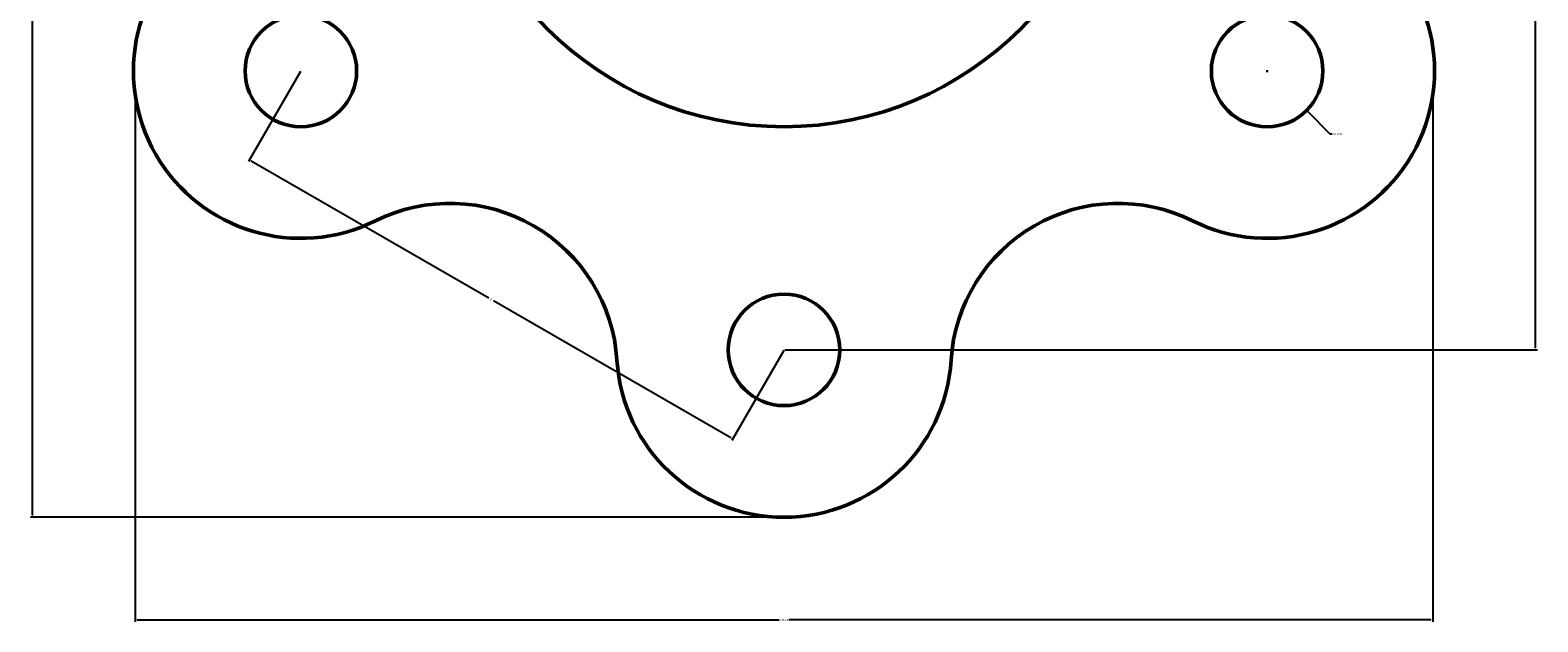
# Model space of a CAD drawing. Units: millimetres. Extents: x 2038 to 2173, y 1596 to 1745.
# Tile 1 of 4: x 2038 to 2173, y 1596 to 1649. Entities that reach past the tile are written whole.
import ezdxf

# ---------------------------------------------------------------- set-up
doc = ezdxf.new("R2010")
doc.units = ezdxf.units.MM
doc.layers.add('M-DIMS', color=2, linetype='Continuous', lineweight=18)
doc.layers.add('M-OUTL', color=7, linetype='Continuous', lineweight=50)
doc.styles.get("Standard").update_dxf_attribs({"font": 'arial.ttf'})
doc.dimstyles.get("Standard").update_dxf_attribs({"dimtxt": 0.18, "dimasz": 0.18, "dimexe": 0.18, "dimexo": 0.0625, "dimgap": 0.09, "dimtad": 0, "dimtih": 1, "dimtoh": 1, "dimdec": 4, "dimzin": 0, "dimdsep": 46, "dimtxsty": 'Standard', "dimcen": 0.09, "dimadec": 0, "dimazin": 0, "dimtfac": 1, "dimtdec": 4, "dimtofl": 0, "dimtmove": 0, "dimatfit": 3, "dimfxl": 1, "dimtolj": 1, "dimtzin": 0, "dimarcsym": 0})

# ---------------------------------------------------------------- blocks, each defined once
blk = doc.blocks.new('*U1')
blk.add_arc((-4.15, 7.97), 15, 243.5573, 356.4427)
blk = doc.blocks.new('*U2')
at = {"layer": 'M-OUTL', "color": 0, "linetype": 'ByBlock', "lineweight": -2, "transparency": 16777216}
for p, rotation in [((2130.6, 1715.07), 300), ((2156.4, 1671.18), 240), ((2054.57, 1670.39), 60.00000000000003), ((2080.37, 1626.5), 120.0000000000001), ((2131.28, 1626.89), 180)]:
    blk.add_blockref('*U1', p, dxfattribs=dict(at, rotation=rotation))
blk.add_blockref('*U1', (2079.69, 1714.68), dxfattribs=at)
blk = doc.blocks.new('FLANGE-LUG-D10')
blk.add_circle((0, 0), 5)
blk.add_arc((0, 0), 15, 3.5573, 176.4427)
blk = doc.blocks.new('*D4')
at = {"layer": 'Defpoints', "color": 0, "transparency": 16777216}
for p in [(2047.33, 1643.69), (2163.64, 1643.69), (2163.64, 1596.58)]:
    blk.add_point(p, dxfattribs=at)
at = {"layer": 'M-DIMS', "color": 0, "lineweight": -2, "transparency": 16777216}
for p, q in [((2047.33, 1643.63), (2047.33, 1596.4)), ((2163.64, 1643.63), (2163.64, 1596.4)), ((2047.51, 1596.58), (2105.05, 1596.58)), ((2163.46, 1596.58), (2105.93, 1596.58))]:
    blk.add_line(p, q, dxfattribs=at)
at = {"layer": 'M-DIMS', "color": 0, "transparency": 16777216}
for points in [[(2047.51, 1596.61), (2047.51, 1596.55), (2047.33, 1596.58)], [(2163.46, 1596.61), (2163.46, 1596.55), (2163.64, 1596.58)]]:
    blk.add_solid(points, dxfattribs=at)
at = {"layer": 'M-DIMS', "color": 0, "transparency": 16777216, "insert": (2105.49, 1596.58), "char_height": 0.18, "attachment_point": 5}
blk.add_mtext('\\A1;116.31', dxfattribs=at)
blk = doc.blocks.new('*D5')
at = {"layer": 'Defpoints', "color": 0, "transparency": 16777216}
for p in [(2038.13, 1735.78), (2105.49, 1735.78), (2105.49, 1605.78)]:
    blk.add_point(p, dxfattribs=at)
at = {"layer": 'M-DIMS', "color": 0, "lineweight": -2, "transparency": 16777216}
for p, q in [((2105.43, 1735.78), (2037.95, 1735.78)), ((2038.13, 1735.6), (2038.13, 1670.97)), ((2038.13, 1605.96), (2038.13, 1670.6)), ((2105.43, 1605.78), (2037.95, 1605.78))]:
    blk.add_line(p, q, dxfattribs=at)
at = {"layer": 'M-DIMS', "color": 0, "transparency": 16777216}
for points in [[(2038.1, 1735.6), (2038.16, 1735.6), (2038.13, 1735.78)], [(2038.1, 1605.96), (2038.16, 1605.96), (2038.13, 1605.78)]]:
    blk.add_solid(points, dxfattribs=at)
at = {"layer": 'M-DIMS', "color": 0, "transparency": 16777216, "insert": (2038.13, 1670.78), "char_height": 0.18, "attachment_point": 5}
blk.add_mtext('\\A1;130', dxfattribs=at)
blk = doc.blocks.new('*D6')
at = {"layer": 'Defpoints', "color": 0, "transparency": 16777216}
for p in [(2105.49, 1720.78), (2172.84, 1720.78), (2105.49, 1620.78)]:
    blk.add_point(p, dxfattribs=at)
at = {"layer": 'M-DIMS', "color": 0, "lineweight": -2, "transparency": 16777216}
for p, q in [((2105.55, 1720.78), (2173.02, 1720.78)), ((2172.84, 1720.6), (2172.84, 1670.97)), ((2172.84, 1620.96), (2172.84, 1670.6)), ((2105.55, 1620.78), (2173.02, 1620.78))]:
    blk.add_line(p, q, dxfattribs=at)
at = {"layer": 'M-DIMS', "color": 0, "transparency": 16777216}
for points in [[(2172.81, 1720.6), (2172.87, 1720.6), (2172.84, 1720.78)], [(2172.81, 1620.96), (2172.87, 1620.96), (2172.84, 1620.78)]]:
    blk.add_solid(points, dxfattribs=at)
at = {"layer": 'M-DIMS', "color": 0, "transparency": 16777216, "insert": (2172.84, 1670.78), "char_height": 0.18, "attachment_point": 5}
blk.add_mtext('\\A1;100', dxfattribs=at)
blk = doc.blocks.new('*D7')
at = {"layer": 'Defpoints', "color": 0, "transparency": 16777216}
for p in [(2062.19, 1645.78), (2057.59, 1637.82), (2105.49, 1620.78)]:
    blk.add_point(p, dxfattribs=at)
at = {"layer": 'M-DIMS', "color": 0, "lineweight": -2, "transparency": 16777216}
for p, q in [((2062.16, 1645.73), (2057.5, 1637.66)), ((2057.74, 1637.73), (2079.02, 1625.44)), ((2100.73, 1612.91), (2079.46, 1625.19)), ((2105.46, 1620.73), (2100.8, 1612.66))]:
    blk.add_line(p, q, dxfattribs=at)
at = {"layer": 'M-DIMS', "color": 0, "transparency": 16777216}
for points in [[(2057.76, 1637.75), (2057.73, 1637.7), (2057.59, 1637.82)], [(2100.75, 1612.93), (2100.72, 1612.88), (2100.89, 1612.82)]]:
    blk.add_solid(points, dxfattribs=at)
at = {"layer": 'M-DIMS', "color": 0, "transparency": 16777216, "insert": (2079.24, 1625.32), "char_height": 0.18, "attachment_point": 5}
blk.add_mtext('\\A1;50', dxfattribs=at)
blk = doc.blocks.new('*D13')
at = {"layer": 'Defpoints', "color": 0, "transparency": 16777216}
for p in [(2145.25, 1649.32), (2152.32, 1642.25)]:
    blk.add_point(p, dxfattribs=at)
at = {"layer": 'M-DIMS', "color": 0, "lineweight": -2, "transparency": 16777216}
for p, q in [((2148.79, 1645.69), (2148.79, 1645.87)), ((2148.7, 1645.78), (2148.88, 1645.78)), ((2154.45, 1640.13), (2152.45, 1642.12)), ((2154.63, 1640.13), (2154.45, 1640.13))]:
    blk.add_line(p, q, dxfattribs=at)
at = {"layer": 'M-DIMS', "color": 0, "transparency": 16777216}
blk.add_solid([(2152.47, 1642.14), (2152.43, 1642.1), (2152.32, 1642.25)], dxfattribs=at)
at = {"layer": 'M-DIMS', "color": 0, "transparency": 16777216, "insert": (2155.13, 1640.13), "char_height": 0.18, "attachment_point": 5}
blk.add_mtext('\\A1;6X ∅10', dxfattribs=at)

msp = doc.modelspace()

# ---------------------------------------------------------------- linework, layer by layer
at = {"layer": 'M-OUTL'}
msp.add_circle((2105.488, 1670.784), 30, dxfattribs=at)

# ---------------------------------------------------------------- block references
msp.add_blockref('*U2', (0, 0), dxfattribs=at)
for p, rotation in [((2062.186, 1645.784), 120.0000000000013), ((2148.789, 1645.784), 239.9999999999991), ((2105.488, 1620.784), 180)]:
    msp.add_blockref('FLANGE-LUG-D10', p, dxfattribs=dict(at, rotation=rotation))

# ---------------------------------------------------------------- dimensions: what is measured, and where the dimension line sits
at = {"layer": 'M-DIMS'}
for base, p1, p2, angle, picture, middle in [((2038.131, 1735.784), (2105.488, 1605.784), (2105.488, 1735.784), 90, '*D5', (2038.131, 1670.784)), ((2172.845, 1720.784), (2105.488, 1620.784), (2105.488, 1720.784), 90, '*D6', (2172.845, 1670.784)), ((2057.586, 1637.817), (2105.488, 1620.784), (2062.186, 1645.784), 150, '*D7', (2079.237, 1625.317))]:
    dim = msp.add_linear_dim(base=base, p1=p1, p2=p2, angle=angle, dimstyle='Standard', override={"dimdec": 0, "dimlfac": 1, "dimrnd": 0, "dimzin": 0, "dimdsep": 46, "dimlunit": 2}, dxfattribs=at)
    dim.commit()
    dim.dimension.update_dxf_attribs({"geometry": picture, "text_midpoint": middle})
dim = msp.add_diameter_dim_2p(p1=(2145.253, 1649.319), p2=(2152.325, 1642.249), text='6X <>', dimstyle='Standard', override={"dimdec": 0, "dimlfac": 1, "dimrnd": 0, "dimzin": 0, "dimdsep": 46, "dimlunit": 2}, dxfattribs=at)
dim.commit()
dim.dimension.update_dxf_attribs({"geometry": '*D13', "text_midpoint": (2155.132, 1640.128), "dimtype": 163})
dim = msp.add_linear_dim(base=(2163.645, 1596.584), p1=(2047.331, 1643.688), p2=(2163.645, 1643.688), dimstyle='Standard', override={"dimdec": 2, "dimlfac": 1, "dimrnd": 0, "dimzin": 0, "dimdsep": 46, "dimlunit": 2}, dxfattribs=at)
dim.commit()
dim.dimension.update_dxf_attribs({"geometry": '*D4', "text_midpoint": (2105.488, 1596.584)})

doc.saveas('drawing.dxf')
